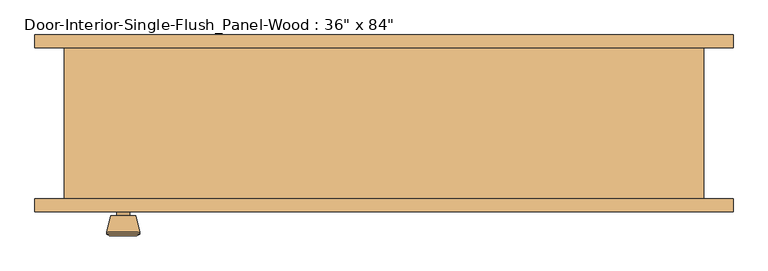
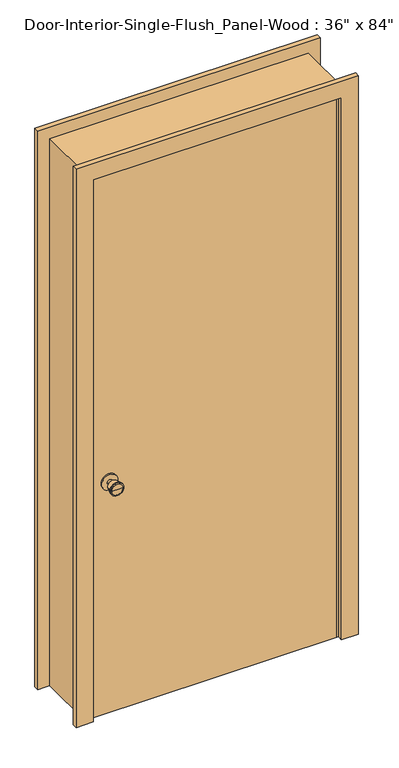
"""IFC4 building model written with IfcOpenShell, lengths in millimetres: door geometry."""

from ifc_helpers import new_model, si_unit, point, frame, frame_2d, origin, origin_with_axes, place, context, project, spatial, polyline, circle_curve, trimmed, segment, composite_curve, outline, extrude, faceted_brep, source, transform, mapped, element, save
from ifc_brep_helpers import plane_surface, cylinder_surface, revolved_surface, advanced_brep


def door_b48525d3(model_context):
    return source(origin(), model_context, "Body", "SolidModel", [
        advanced_brep(
        [(-393.7, -70.2, 914.4), (-403.7, -70.2, 914.4), (-383.7, -70.2, 914.4), (-373.2241324, -21.2, 914.4), (-414.1758676, -21.2, 914.4), (-393.7, -21.2, 914.4), (-368.7, -23.0278681, 914.4), (-418.7, -23.0278681, 914.4), (-368.7, -26.4915463, 914.4), (-418.7, -26.4915463, 914.4), (-375.063764, -51.2, 914.4), (-412.336236, -51.2, 914.4), (-383.7, -51.2, 914.4), (-403.7, -51.2, 914.4)],
        [
            (0, 1),
            (1, 2, circle_curve(frame((-393.7, -70.2, 914.4), z_axis=(0.0, -1.0, 0.0), x_axis=(-1.0, 0.0, 0.0)), 10.0)),
            (2, 0),
            (2, 1, circle_curve(frame((-393.7, -70.2, 914.4), z_axis=(0.0, -1.0, 0.0), x_axis=(-1.0, 0.0, 0.0)), 10.0)),
            (3, 4, circle_curve(frame((-393.7, -21.2, 914.4), z_axis=(0.0, 1.0, 0.0), x_axis=(-1.0, 0.0, 0.0)), 20.4758676)),
            (4, 5),
            (5, 3),
            (4, 3, circle_curve(frame((-393.7, -21.2, 914.4), z_axis=(0.0, 1.0, 0.0), x_axis=(-1.0, 0.0, 0.0)), 20.4758676)),
            (6, 7, circle_curve(frame((-393.7, -23.0278681, 914.4), z_axis=(0.0, 1.0, 0.0), x_axis=(-1.0, 0.0, 0.0)), 25.0)),
            (7, 4),
            (3, 6),
            (7, 6, circle_curve(frame((-393.7, -23.0278681, 914.4), z_axis=(0.0, 1.0, 0.0), x_axis=(-1.0, 0.0, 0.0)), 25.0)),
            (8, 9, circle_curve(frame((-393.7, -26.4915463, 914.4), z_axis=(0.0, 1.0, 0.0), x_axis=(-1.0, 0.0, 0.0)), 25.0)),
            (9, 7),
            (6, 8),
            (9, 8, circle_curve(frame((-393.7, -26.4915463, 914.4), z_axis=(0.0, 1.0, 0.0), x_axis=(-1.0, 0.0, 0.0)), 25.0)),
            (10, 11, circle_curve(frame((-393.7, -51.2, 914.4), z_axis=(0.0, 1.0, 0.0), x_axis=(-1.0, 0.0, 0.0)), 18.636236)),
            (11, 9),
            (8, 10),
            (11, 10, circle_curve(frame((-393.7, -51.2, 914.4), z_axis=(0.0, 1.0, 0.0), x_axis=(-1.0, 0.0, 0.0)), 18.636236)),
            (12, 13, circle_curve(frame((-393.7, -51.2, 914.4), z_axis=(0.0, 1.0, 0.0), x_axis=(-1.0, 0.0, 0.0)), 10.0)),
            (13, 11),
            (10, 12),
            (13, 12, circle_curve(frame((-393.7, -51.2, 914.4), z_axis=(0.0, 1.0, 0.0), x_axis=(-1.0, 0.0, 0.0)), 10.0)),
            (1, 13),
            (12, 2),
        ],
        [
            plane_surface(frame((-393.7, -70.2, 914.4), z_axis=(0.0, -1.0, 0.0), x_axis=(-1.0, 0.0, 0.0))),
            plane_surface(frame((-393.7, -21.2, 914.4), z_axis=(0.0, 1.0, 0.0), x_axis=(-1.0, 0.0, 0.0))),
            revolved_surface(polyline([(-414.1758676, -21.2, 914.4), (-418.7, -23.0278681, 914.4)]), (-393.7, -70.2, 914.4), (0.0, -1.0, 0.0)),
            cylinder_surface(frame((-393.7, -70.2, 914.4), z_axis=(0.0, -1.0, 0.0), x_axis=(-1.0, 0.0, 0.0)), 25.0),
            revolved_surface(polyline([(-418.7, -26.4915463, 914.4), (-412.336236, -51.2, 914.4)]), (-393.7, -70.2, 914.4), (0.0, -1.0, 0.0)),
            plane_surface(frame((-393.7, -51.2, 914.4), z_axis=(0.0, -1.0, 0.0), x_axis=(-1.0, 0.0, 0.0))),
            cylinder_surface(frame((-393.7, -70.2, 914.4), z_axis=(0.0, -1.0, 0.0), x_axis=(-1.0, 0.0, 0.0)), 10.0),
        ],
        [
            (0, [[1, 2, 3]]),
            (0, [[-3, 4, -1]]),
            (1, [[5, 6, 7]]),
            (1, [[8, -7, -6]]),
            (2, [[9, 10, -5, 11]]),
            (2, [[12, -11, -8, -10]]),
            (3, [[13, 14, -9, 15]]),
            (3, [[16, -15, -12, -14]]),
            (4, [[17, 18, -13, 19]]),
            (4, [[20, -19, -16, -18]]),
            (5, [[21, 22, -17, 23]]),
            (5, [[24, -23, -20, -22]]),
            (6, [[-2, 25, -21, 26]]),
            (6, [[-4, -26, -24, -25]]),
        ],
    ),
        extrude(outline(composite_curve([segment(trimmed(circle_curve(frame_2d((914.4, -393.7)), 30.0), [point((914.4, -423.7))], [point((914.4, -363.7))], False, "CARTESIAN"), True, "CONTINUOUS"), segment(trimmed(circle_curve(frame_2d((914.4, -393.7)), 30.0), [point((914.4, -363.7))], [point((914.4, -423.7))], False, "CARTESIAN"), True, "CONTINUOUS")], self_intersect=False)), frame((0.0, -76.2, 0.0), z_axis=(0.0, 1.0, 0.0), x_axis=(0.0, 0.0, 1.0)), (0.0, 0.0, 1.0), 6.0),
        advanced_brep(
        [(-393.7, -117.125, 914.4), (-383.7, -117.125, 914.4), (-403.7, -117.125, 914.4), (-373.2241324, -166.125, 914.4), (-393.7, -166.125, 914.4), (-414.1758676, -166.125, 914.4), (-368.7, -164.2971319, 914.4), (-418.7, -164.2971319, 914.4), (-368.7, -160.8334537, 914.4), (-418.7, -160.8334537, 914.4), (-375.063764, -136.125, 914.4), (-412.336236, -136.125, 914.4), (-383.7, -136.125, 914.4), (-403.7, -136.125, 914.4)],
        [
            (0, 1),
            (1, 2, circle_curve(frame((-393.7, -117.125, 914.4), z_axis=(0.0, 1.0, 0.0), x_axis=(-1.0, 0.0, 0.0)), 10.0)),
            (2, 0),
            (2, 1, circle_curve(frame((-393.7, -117.125, 914.4), z_axis=(0.0, 1.0, 0.0), x_axis=(-1.0, 0.0, 0.0)), 10.0)),
            (3, 4),
            (4, 5),
            (5, 3, circle_curve(frame((-393.7, -166.125, 914.4), z_axis=(0.0, -1.0, 0.0), x_axis=(-1.0, 0.0, 0.0)), 20.4758676)),
            (3, 5, circle_curve(frame((-393.7, -166.125, 914.4), z_axis=(0.0, -1.0, 0.0), x_axis=(-1.0, 0.0, 0.0)), 20.4758676)),
            (6, 3),
            (5, 7),
            (7, 6, circle_curve(frame((-393.7, -164.2971319, 914.4), z_axis=(0.0, -1.0, 0.0), x_axis=(-1.0, 0.0, 0.0)), 25.0)),
            (6, 7, circle_curve(frame((-393.7, -164.2971319, 914.4), z_axis=(0.0, -1.0, 0.0), x_axis=(-1.0, 0.0, 0.0)), 25.0)),
            (8, 6),
            (7, 9),
            (9, 8, circle_curve(frame((-393.7, -160.8334537, 914.4), z_axis=(0.0, -1.0, 0.0), x_axis=(-1.0, 0.0, 0.0)), 25.0)),
            (8, 9, circle_curve(frame((-393.7, -160.8334537, 914.4), z_axis=(0.0, -1.0, 0.0), x_axis=(-1.0, 0.0, 0.0)), 25.0)),
            (10, 8),
            (9, 11),
            (11, 10, circle_curve(frame((-393.7, -136.125, 914.4), z_axis=(0.0, -1.0, 0.0), x_axis=(-1.0, 0.0, 0.0)), 18.636236)),
            (10, 11, circle_curve(frame((-393.7, -136.125, 914.4), z_axis=(0.0, -1.0, 0.0), x_axis=(-1.0, 0.0, 0.0)), 18.636236)),
            (12, 10),
            (11, 13),
            (13, 12, circle_curve(frame((-393.7, -136.125, 914.4), z_axis=(0.0, -1.0, 0.0), x_axis=(-1.0, 0.0, 0.0)), 10.0)),
            (12, 13, circle_curve(frame((-393.7, -136.125, 914.4), z_axis=(0.0, -1.0, 0.0), x_axis=(-1.0, 0.0, 0.0)), 10.0)),
            (1, 12),
            (13, 2),
        ],
        [
            plane_surface(frame((-393.7, -117.125, 914.4), z_axis=(0.0, 1.0, 0.0), x_axis=(-1.0, 0.0, 0.0))),
            plane_surface(frame((-393.7, -166.125, 914.4), z_axis=(0.0, -1.0, 0.0), x_axis=(-1.0, 0.0, 0.0))),
            revolved_surface(polyline([(-414.1758676, -166.125, 914.4), (-418.7, -164.2971319, 914.4)]), (-393.7, -117.125, 914.4), (0.0, 1.0, 0.0)),
            cylinder_surface(frame((-393.7, -117.125, 914.4), z_axis=(0.0, 1.0, 0.0), x_axis=(-1.0, 0.0, 0.0)), 25.0),
            revolved_surface(polyline([(-418.7, -160.8334537, 914.4), (-412.336236, -136.125, 914.4)]), (-393.7, -117.125, 914.4), (0.0, 1.0, 0.0)),
            plane_surface(frame((-393.7, -136.125, 914.4), z_axis=(0.0, 1.0, 0.0), x_axis=(-1.0, 0.0, 0.0))),
            cylinder_surface(frame((-393.7, -117.125, 914.4), z_axis=(0.0, 1.0, 0.0), x_axis=(-1.0, 0.0, 0.0)), 10.0),
        ],
        [
            (0, [[1, 2, 3]]),
            (0, [[-3, 4, -1]]),
            (1, [[5, 6, 7]]),
            (1, [[-6, -5, 8]]),
            (2, [[9, -7, 10, 11]]),
            (2, [[-10, -8, -9, 12]]),
            (3, [[13, -11, 14, 15]]),
            (3, [[-14, -12, -13, 16]]),
            (4, [[17, -15, 18, 19]]),
            (4, [[-18, -16, -17, 20]]),
            (5, [[21, -19, 22, 23]]),
            (5, [[-22, -20, -21, 24]]),
            (6, [[25, -23, 26, -2]]),
            (6, [[-26, -24, -25, -4]]),
        ],
    ),
        extrude(outline(composite_curve([segment(trimmed(circle_curve(frame_2d((914.4, -393.7)), 30.0), [point((914.4, -423.7))], [point((914.4, -363.7))], False, "CARTESIAN"), True, "CONTINUOUS"), segment(trimmed(circle_curve(frame_2d((914.4, -393.7)), 30.0), [point((914.4, -363.7))], [point((914.4, -423.7))], False, "CARTESIAN"), True, "CONTINUOUS")], self_intersect=False)), frame((0.0, -117.125, 0.0), z_axis=(0.0, 1.0, 0.0), x_axis=(0.0, 0.0, 1.0)), (0.0, 0.0, 1.0), 6.0),
        faceted_brep([(482.6, -111.125, 0.0), (457.2, -111.125, 0.0), (457.2, -76.2, 0.0), (444.5, -76.2, 0.0), (444.5, -41.275, 0.0), (457.2, -41.275, 0.0), (457.2, 117.475, 0.0), (482.6, 117.475, 0.0), (482.6, 117.475, 2159.0), (482.6, -111.125, 2159.0), (457.2, 117.475, 2133.6), (-457.2, 117.475, 2133.6), (-457.2, 117.475, 0.0), (-482.6, 117.475, 0.0), (-482.6, 117.475, 2159.0), (457.2, -41.275, 2133.6), (444.5, -41.275, 2120.9), (-444.5, -41.275, 2120.9), (-444.5, -41.275, 0.0), (-457.2, -41.275, 0.0), (-457.2, -41.275, 2133.6), (444.5, -76.2, 2120.9), (457.2, -76.2, 2133.6), (-457.2, -76.2, 2133.6), (-457.2, -76.2, 0.0), (-444.5, -76.2, 0.0), (-444.5, -76.2, 2120.9), (457.2, -111.125, 2133.6), (-482.6, -111.125, 2159.0), (-482.6, -111.125, 0.0), (-457.2, -111.125, 0.0), (-457.2, -111.125, 2133.6)], [[[0, 1, 2, 3, 4, 5, 6, 7]], [[7, 8, 9, 0]], [[6, 10, 11, 12, 13, 14, 8, 7]], [[5, 15, 10, 6]], [[4, 16, 17, 18, 19, 20, 15, 5]], [[3, 21, 16, 4]], [[2, 22, 23, 24, 25, 26, 21, 3]], [[1, 27, 22, 2]], [[0, 9, 28, 29, 30, 31, 27, 1]], [[8, 14, 28, 9]], [[15, 20, 11, 10]], [[21, 26, 17, 16]], [[27, 31, 23, 22]], [[29, 13, 12, 19, 18, 25, 24, 30]], [[14, 13, 29, 28]], [[20, 19, 12, 11]], [[26, 25, 18, 17]], [[31, 30, 24, 23]]]),
        extrude(outline(polyline([(457.2, -76.2), (457.2, -111.125), (-457.2, -111.125), (-457.2, -76.2), (457.2, -76.2)])), origin_with_axes(), (0.0, 0.0, 1.0), 2133.6),
        extrude(outline(polyline([(0.0, 527.05), (2203.45, 527.05), (2203.45, -527.05), (0.0, -527.05), (0.0, -463.55), (2139.95, -463.55), (2139.95, 463.55), (0.0, 463.55), (0.0, 527.05)])), frame((0.0, -130.175, 0.0), z_axis=(0.0, 1.0, 0.0), x_axis=(0.0, 0.0, 1.0)), (0.0, 0.0, 1.0), 19.05),
        extrude(outline(polyline([(0.0, 527.05), (2203.45, 527.05), (2203.45, -527.05), (0.0, -527.05), (0.0, -463.55), (2139.95, -463.55), (2139.95, 463.55), (0.0, 463.55), (0.0, 527.05)])), frame((0.0, 117.475, 0.0), z_axis=(0.0, 1.0, 0.0), x_axis=(0.0, 0.0, 1.0)), (0.0, 0.0, 1.0), 19.05),
    ])


if __name__ == "__main__":
    model = new_model("IFC4")
    model_context = context("Model", 3, world=origin())
    ifc_project = project(units=[si_unit("LENGTHUNIT", "METRE", prefix="MILLI")], contexts=[model_context])
    site = spatial("IfcSite", under=ifc_project)
    building = spatial("IfcBuilding", under=site)
    placement = place(None, origin())
    door_shape = door_b48525d3(model_context)
    element("IfcDoor", 1, ObjectType="Door-Interior-Single-Flush_Panel-Wood : 36\" x 84\"", at=placement, inside=building, context=model_context, shape_type="MappedRepresentation", body=[
        mapped(door_shape, transform((0.0, 0.0, 0.0), x_axis=(1.0, 0.0, 0.0), y_axis=(0.0, 1.0, 0.0), z_axis=(0.0, 0.0, 1.0))),
    ])
    save(model, "model.ifc")

# Revit data of these elements
# Type "Door-Interior-Single-Flush_Panel-Wood : 36\" x 84\""
#   Type Mark = "12"
#   Analytic Construction = "Wooden"
#   Thickness = 0' - 1 3/8"
#   Thermal Resistance (R) = 2.5876 (h·ft²·°F)/BTU
#   Swing Angle [instance default] = 90.00°
#   Rough Width = 3' - 2"
#   Rough Height = 7' - 1"
#   Height = 7' - 0"
#   Width = 3' - 0"
#   Heat Transfer Coefficient (U) = 0.3865 BTU/(h·ft²·°F)
#   Trim Material = Cherry
#   Panel Material = Cherry
#   Frame Material = Cherry
#   Door Handle Material = Aluminum
#   Visual Light Transmittance = 0
#   Solar Heat Gain Coefficient = 0
#   Wall Closure = (empty or 0)
#   Function = (empty or 0)
# Element 1 (IfcDoor, "Door-Interior-Single-Flush_Panel-Wood : 36\" x 84\"")
#   Materials on its faces: "Cherry", "Aluminum"
# Materials
#   "Cherry": class "Wood", colour RGB 226 177 128, transparency 0, Description = "Prunus Serotina", Cost = 0
#   "Aluminum": class "Metal", colour RGB 247 247 247, transparency 0, Description = "Aluminum 6061", Cost = 0
